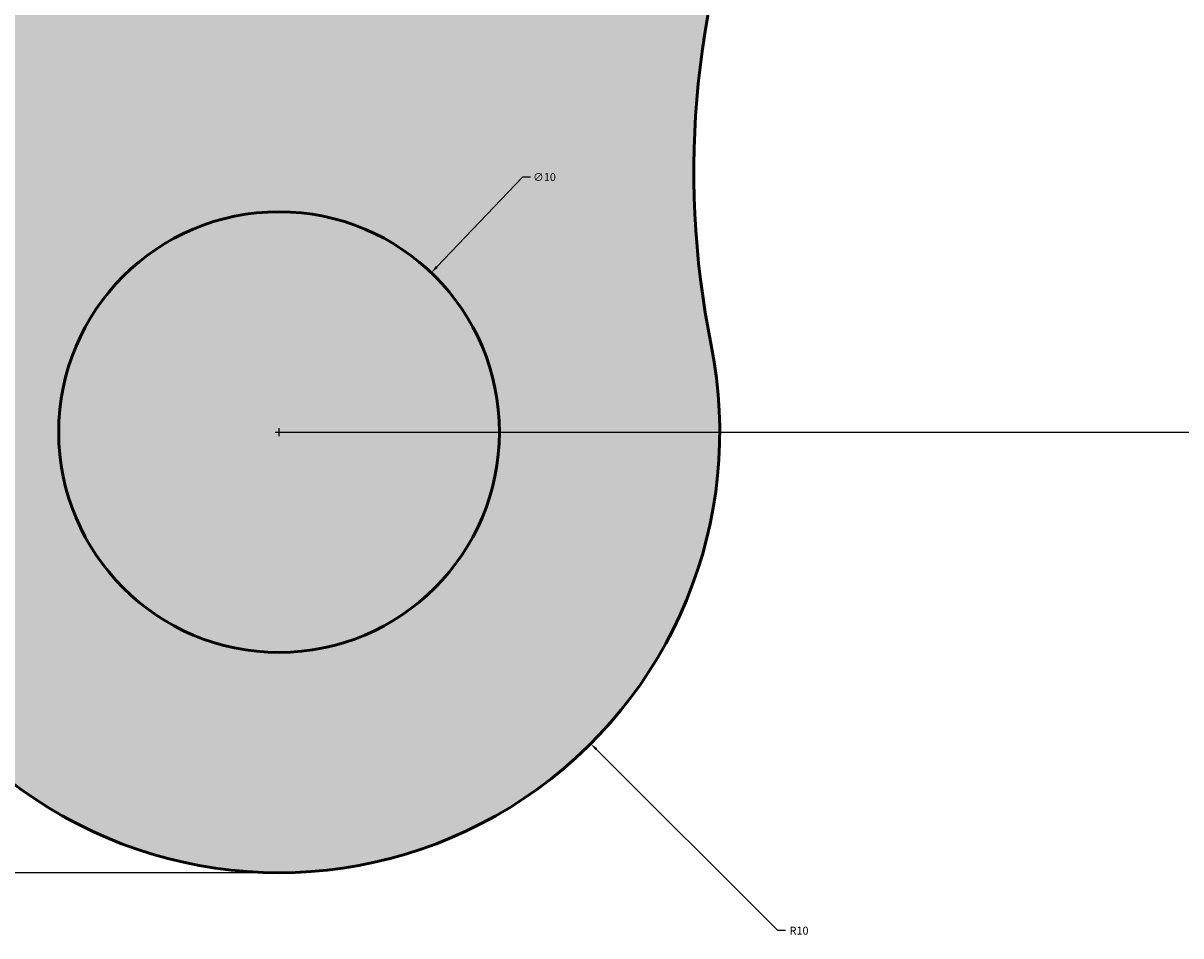
# Model space of a CAD drawing. Units: inches. Extents: x -13 to 107, y -48 to 102.
# Tile 2 of 13: x 22 to 48, y -48 to -27. Entities that reach past the tile are written whole.
import ezdxf

# ---------------------------------------------------------------- set-up
doc = ezdxf.new("R2010")
doc.units = ezdxf.units.IN
doc.header["$MEASUREMENT"] = 0
for name, color, linetype, lineweight in [('M-DIMS', 2, 'Continuous', 18), ('M-HATC', 8, 'Continuous', 18), ('M-OUTL', 7, 'Continuous', 50)]:
    doc.layers.add(name, color=color, linetype=linetype, lineweight=lineweight)
doc.styles.get("Standard").update_dxf_attribs({"font": 'arial.ttf'})
doc.dimstyles.get("Standard").update_dxf_attribs({"dimtxt": 0.18, "dimasz": 0.18, "dimexe": 0.18, "dimexo": 0.0625, "dimgap": 0.09, "dimtad": 0, "dimtih": 1, "dimtoh": 1, "dimdec": 4, "dimzin": 0, "dimdsep": 46, "dimtxsty": 'Standard', "dimcen": 0.09, "dimadec": 0, "dimazin": 0, "dimtfac": 1, "dimtdec": 4, "dimtofl": 0, "dimtmove": 0, "dimatfit": 3, "dimfxl": 1, "dimtolj": 1, "dimtzin": 0, "dimarcsym": 0})

# ---------------------------------------------------------------- blocks, each defined once
blk = doc.blocks.new('*D2')
at = {"layer": 'Defpoints', "color": 0, "transparency": 16777216}
for p in [(-12.585, 94.408), (27.547, 94.408), (27.547, -46.592)]:
    blk.add_point(p, dxfattribs=at)
at = {"layer": 'M-DIMS', "color": 0, "lineweight": -2, "transparency": 16777216}
for p, q in [((27.484, 94.408), (-12.765, 94.408)), ((-12.585, 94.228), (-12.585, 24.088)), ((-12.585, -46.412), (-12.585, 23.727)), ((27.484, -46.592), (-12.765, -46.592))]:
    blk.add_line(p, q, dxfattribs=at)
at = {"layer": 'M-DIMS', "color": 0, "transparency": 16777216}
for points in [[(-12.615, 94.228), (-12.555, 94.228), (-12.585, 94.408)], [(-12.615, -46.412), (-12.555, -46.412), (-12.585, -46.592)]]:
    blk.add_solid(points, dxfattribs=at)
at = {"layer": 'M-DIMS', "color": 0, "transparency": 16777216, "insert": (-12.585, 23.908), "char_height": 0.18, "attachment_point": 5}
blk.add_mtext('\\A1;141', dxfattribs=at)
blk = doc.blocks.new('*D3')
at = {"layer": 'Defpoints', "color": 0, "transparency": 16777216}
for p in [(27.547, 13.408), (67.679, 13.408), (27.547, -36.592)]:
    blk.add_point(p, dxfattribs=at)
at = {"layer": 'M-DIMS', "color": 0, "lineweight": -2, "transparency": 16777216}
for p, q in [((27.609, 13.408), (67.859, 13.408)), ((67.679, 13.228), (67.679, -11.41)), ((67.679, -36.412), (67.679, -11.774)), ((27.609, -36.592), (67.859, -36.592))]:
    blk.add_line(p, q, dxfattribs=at)
at = {"layer": 'M-DIMS', "color": 0, "transparency": 16777216}
for points in [[(67.649, 13.228), (67.709, 13.228), (67.679, 13.408)], [(67.649, -36.412), (67.709, -36.412), (67.679, -36.592)]]:
    blk.add_solid(points, dxfattribs=at)
at = {"layer": 'M-DIMS', "color": 0, "transparency": 16777216, "insert": (67.679, -11.592), "char_height": 0.18, "attachment_point": 5}
blk.add_mtext('\\A1;50', dxfattribs=at)
blk = doc.blocks.new('*D11')
at = {"layer": 'Defpoints', "color": 0, "transparency": 16777216}
for p in [(38.592, -22.767), (56.959, -30.682)]:
    blk.add_point(p, dxfattribs=at)
at = {"layer": 'M-DIMS', "color": 0, "lineweight": -2, "transparency": 16777216}
for p, q in [((27.392, -18.018), (27.572, -18.018)), ((27.572, -18.018), (38.427, -22.696)), ((56.869, -30.682), (57.049, -30.682)), ((56.959, -30.772), (56.959, -30.592))]:
    blk.add_line(p, q, dxfattribs=at)
at = {"layer": 'M-DIMS', "color": 0, "transparency": 16777216}
blk.add_solid([(38.438, -22.668), (38.415, -22.724), (38.592, -22.767)], dxfattribs=at)
at = {"layer": 'M-DIMS', "color": 0, "transparency": 16777216, "insert": (26.892, -18.018), "char_height": 0.18, "attachment_point": 5}
blk.add_mtext('\\A1;2X R20', dxfattribs=at)
blk = doc.blocks.new('*D12')
at = {"layer": 'Defpoints', "color": 0, "transparency": 16777216}
for p in [(27.547, -36.592), (34.618, -43.663)]:
    blk.add_point(p, dxfattribs=at)
at = {"layer": 'M-DIMS', "color": 0, "lineweight": -2, "transparency": 16777216}
for p, q in [((27.547, -36.682), (27.547, -36.502)), ((27.457, -36.592), (27.637, -36.592)), ((38.861, -47.906), (34.745, -43.79)), ((39.041, -47.906), (38.861, -47.906))]:
    blk.add_line(p, q, dxfattribs=at)
at = {"layer": 'M-DIMS', "color": 0, "transparency": 16777216}
blk.add_solid([(34.767, -43.769), (34.724, -43.812), (34.618, -43.663)], dxfattribs=at)
at = {"layer": 'M-DIMS', "color": 0, "transparency": 16777216, "insert": (39.346, -47.906), "char_height": 0.18, "attachment_point": 5}
blk.add_mtext('\\A1;R10', dxfattribs=at)
blk = doc.blocks.new('*D13')
at = {"layer": 'Defpoints', "color": 0, "transparency": 16777216}
for p in [(31, -32.976), (24.094, -40.208)]:
    blk.add_point(p, dxfattribs=at)
at = {"layer": 'M-DIMS', "color": 0, "lineweight": -2, "transparency": 16777216}
for p, q in [((33.072, -30.806), (31.124, -32.846)), ((33.252, -30.806), (33.072, -30.806)), ((27.547, -36.682), (27.547, -36.502)), ((27.457, -36.592), (27.637, -36.592))]:
    blk.add_line(p, q, dxfattribs=at)
at = {"layer": 'M-DIMS', "color": 0, "transparency": 16777216}
blk.add_solid([(31.103, -32.825), (31.146, -32.867), (31, -32.976)], dxfattribs=at)
at = {"layer": 'M-DIMS', "color": 0, "transparency": 16777216, "insert": (33.568, -30.806), "char_height": 0.18, "attachment_point": 5}
blk.add_mtext('\\A1;∅10', dxfattribs=at)

msp = doc.modelspace()

# ---------------------------------------------------------------- hatches: boundary and pattern name
at = {"layer": 'M-HATC'}
h = msp.add_hatch(color=256, dxfattribs=at)
h.set_gradient(color1=(88, 186, 72), color2=(241, 235, 31), tint=1)
h.paths.add_polyline_path([(45.86, -14.044, 0.420873), (54.577, 32.339, -0.184081), (43.437, 76.537, 1.124637), (11.657, 76.537, -0.184081), (0.517, 32.339, 0.420873), (9.234, -14.044, -0.304084), (17.743, -34.622, 1.220926), (37.351, -34.622, -0.304084)])
h.paths.add_polyline_path([(33.479, -5.692, 0.859727), (21.615, -5.692, -0.111692), (13.972, -1.28, 0.859727), (8.04, 8.995, -0.111692), (8.04, 17.82, 0.859727), (13.972, 28.095, -0.111692), (21.615, 32.508, 0.859727), (33.479, 32.508, -0.111692), (41.122, 28.095, 0.859727), (47.054, 17.82, -0.111692), (47.054, 8.995, 0.859727), (41.122, -1.28, -0.111692)], flags=16)
h.paths.add_polyline_path([(32.547, -36.592, -1), (22.547, -36.592, -1)], flags=16)
h.paths.add_polyline_path([(17.547, 78.408, -1), (37.547, 78.408, -1)], flags=16)
h = msp.add_hatch(color=256, dxfattribs=at)
h.set_gradient(color1=(0, 0, 255), tint=1)
h.paths.add_polyline_path([(47.054, 8.995, 0.111692), (47.054, 17.82, -0.859727), (41.122, 28.095, 0.111692), (33.479, 32.508, -0.859727), (21.615, 32.508, 0.111692), (13.972, 28.095, -0.859727), (8.04, 17.82, 0.111692), (8.04, 8.995, -0.859727), (13.972, -1.28, 0.111692), (21.615, -5.692, -0.859727), (33.479, -5.692, 0.111692), (41.122, -1.28, -0.859727)])
h.paths.add_polyline_path([(37.547, 78.408, 1), (17.547, 78.408, 1)])
h.paths.add_polyline_path([(32.547, -36.592, 1), (22.547, -36.592, 1)])

# ---------------------------------------------------------------- linework, layer by layer
at = {"layer": 'M-OUTL'}
msp.add_circle((27.547, -36.592), 5, dxfattribs=at)
for centre, radius, start, end in [((56.959, -30.682), 20, 123.707, 191.3616), ((27.547, -36.592), 10, 168.6384, 11.3616)]:
    msp.add_arc(centre, radius, start, end, dxfattribs=at)

# ---------------------------------------------------------------- dimensions: what is measured, and where the dimension line sits
at = {"layer": 'M-DIMS'}
for base, p1, p2, picture, middle in [((-12.585, 94.408), (27.547, -46.592), (27.547, 94.408), '*D2', (-12.585, 23.908)), ((67.679, 13.408), (27.547, -36.592), (27.547, 13.408), '*D3', (67.679, -11.592))]:
    dim = msp.add_linear_dim(base=base, p1=p1, p2=p2, angle=90, dimstyle='Standard', override={"dimdec": 0, "dimlfac": 1, "dimrnd": 0, "dimzin": 0, "dimdsep": 46, "dimlunit": 2}, dxfattribs=at)
    dim.commit()
    dim.dimension.update_dxf_attribs({"geometry": picture, "text_midpoint": middle})
dim = msp.add_radius_dim(center=(56.959, -30.682), mpoint=(38.592, -22.767), text='2X <>', dimstyle='Standard', override={"dimdec": 0, "dimlfac": 1, "dimrnd": 0, "dimzin": 0, "dimdsep": 46, "dimlunit": 2}, dxfattribs=at)
dim.commit()
dim.dimension.update_dxf_attribs({"geometry": '*D11', "text_midpoint": (26.892, -18.018), "dimtype": 164})
dim = msp.add_diameter_dim_2p(p1=(24.094, -40.208), p2=(31, -32.976), dimstyle='Standard', override={"dimdec": 0, "dimlfac": 1, "dimrnd": 0, "dimzin": 0, "dimdsep": 46, "dimlunit": 2}, dxfattribs=at)
dim.commit()
dim.dimension.update_dxf_attribs({"geometry": '*D13', "text_midpoint": (33.568, -30.806), "dimtype": 163})
dim = msp.add_radius_dim(center=(27.547, -36.592), mpoint=(34.618, -43.663), dimstyle='Standard', override={"dimdec": 0, "dimlfac": 1, "dimrnd": 0, "dimzin": 0, "dimdsep": 46, "dimlunit": 2}, dxfattribs=at)
dim.commit()
dim.dimension.update_dxf_attribs({"geometry": '*D12', "text_midpoint": (39.346, -47.906), "dimtype": 164})

doc.saveas('drawing.dxf')
